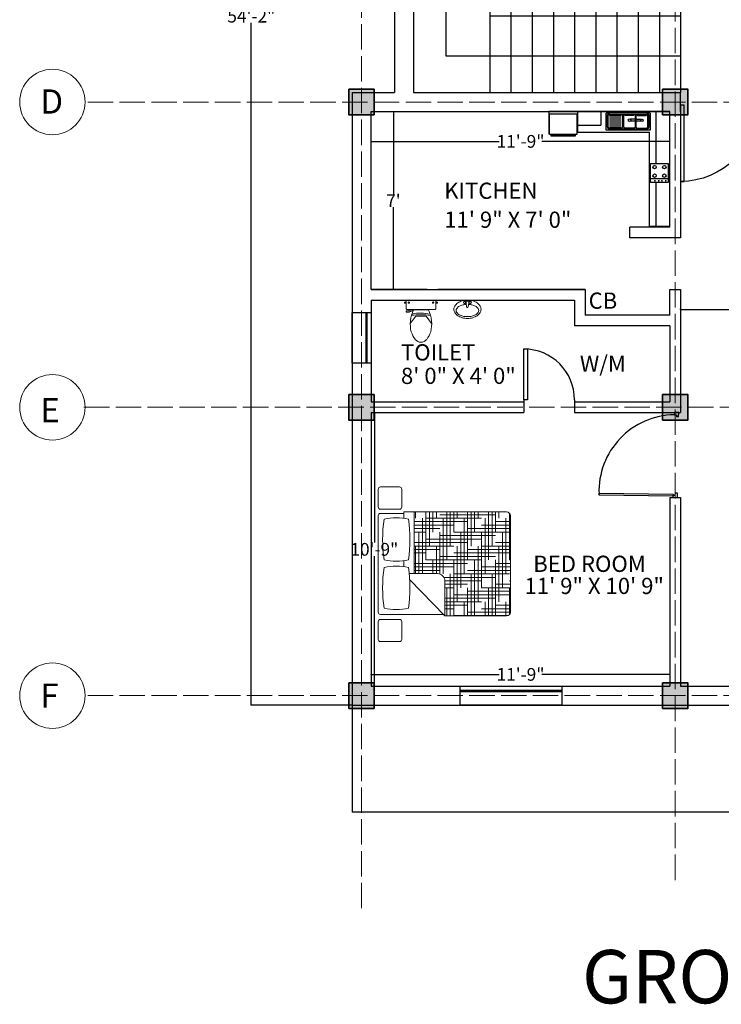
# Model space of a CAD drawing. Units: inches. Extents: x -113 to 5399, y -1393 to 3302.
# Tile 31 of 40: x 3074 to 3405, y 2439 to 2903. Entities that reach past the tile are written whole.
import ezdxf

# ---------------------------------------------------------------- set-up
doc = ezdxf.new("R2010")
doc.units = ezdxf.units.IN
doc.header["$MEASUREMENT"] = 0
doc.linetypes.add('ACAD_ISO02W100', pattern=[15, 12, -3])
for name, color, linetype, lineweight in [('A-ANNO-DIMS', 254, 'Continuous', 18), ('A-ANNO-TEXT', 7, 'Continuous', 25), ('A-AREA-IDEN', 4, 'Continuous', 18), ('A-COLS', 7, 'Continuous', 35), ('A-FLOR-CASE', 8, 'Continuous', 18), ('A-FLOR-FIXT', 8, 'Continuous', 18), ('A-GRID-IDEN', 7, 'Continuous', 18), ('doors', 2, 'Continuous', 25), ('DT TEXT', 4, 'Continuous', 18), ('furniture', 131, 'Continuous', 18), ('GRIDS', 7, 'ACAD_ISO02W100', 13), ('stairs', 210, 'Continuous', 25), ('walls', 1, 'Continuous', 25), ('windows', 3, 'Continuous', 25)]:
    doc.layers.add(name, color=color, linetype=linetype, lineweight=lineweight)
doc.layers.add('TEFRIŞ', color=11, linetype='Continuous')
doc.styles.get("Standard").update_dxf_attribs({"font": 'arial.ttf'})
doc.dimstyles.get("Standard").update_dxf_attribs({"dimtxt": 6, "dimasz": 0.18, "dimexe": 0.18, "dimexo": 0.0625, "dimgap": 0.09, "dimtad": 0, "dimtih": 1, "dimtoh": 1, "dimdec": 1, "dimzin": 0, "dimdsep": 46, "dimlunit": 4, "dimtxsty": 'Standard', "dimblk": 'ARCHTICK', "dimcen": 0.09, "dimadec": 0, "dimazin": 0, "dimtfac": 1, "dimtdec": 1, "dimtofl": 0, "dimtmove": 0, "dimatfit": 3, "dimfxl": 1, "dimtolj": 1, "dimtzin": 0, "dimarcsym": 0})

# ---------------------------------------------------------------- blocks, each defined once
blk = doc.blocks.new('*U2')
for p, q in [((0, 0), (0, -6)), ((24, 0), (24, -6))]:
    blk.add_line(p, q)
blk.add_lwpolyline([(0, 0), (0, 24), (1.75, 24), (1.75, 0)], close=True)
blk.add_arc((0, 0), 24, 0, 90)
blk = doc.blocks.new('*U3')
for p, q in [((0, 0), (0, -6)), ((36, 0), (36, -6))]:
    blk.add_line(p, q)
blk.add_lwpolyline([(0, 0), (0, 36), (1.75, 36), (1.75, 0)], close=True)
blk.add_arc((0, 0), 36, 0, 90)
blk = doc.blocks.new('*X4')
at = {"color": 0}
for p, q in [((4.359, 18.562), (4.359, 18.646)), ((4.5, 18), (4.5, 18.646)), ((4.547, 18.188), (4.547, 18.646)), ((4.594, 18.375), (4.594, 18.646)), ((4.641, 18.562), (4.641, 18.646)), ((4.687, 18.609), (5.437, 18.609)), ((4.781, 18), (4.781, 18.646)), ((4.828, 18.188), (4.828, 18.646)), ((4.875, 18.375), (4.875, 18.646)), ((4.922, 18.562), (4.922, 18.646)), ((5.062, 18), (5.062, 18.646)), ((5.109, 18.188), (5.109, 18.646)), ((5.156, 18.375), (5.156, 18.646)), ((5.203, 18.562), (5.203, 18.646)), ((5.344, 18), (5.344, 18.646)), ((5.391, 18.188), (5.391, 18.646)), ((5.437, 18.375), (5.437, 18.646)), ((5.484, 18.562), (5.484, 18.646)), ((5.625, 18), (5.625, 18.629)), ((4.34, 18.516), (5.062, 18.516)), ((4.34, 18.469), (4.875, 18.469)), ((4.453, 17.817), (4.453, 18.562)), ((4.5, 18.562), (5.25, 18.562)), ((4.734, 17.812), (4.734, 18.562)), ((5.016, 17.812), (5.016, 18.562)), ((5.25, 18.469), (5.637, 18.469)), ((5.297, 17.812), (5.297, 18.562)), ((5.437, 18.516), (5.637, 18.516)), ((5.578, 17.812), (5.578, 18.562)), ((5.625, 18.562), (5.637, 18.562)), ((4.34, 18.422), (4.687, 18.422)), ((4.34, 18.375), (4.5, 18.375)), ((4.406, 17.817), (4.406, 18.375)), ((4.687, 18.328), (5.437, 18.328)), ((4.687, 17.811), (4.687, 18.375)), ((4.875, 18.375), (5.625, 18.375)), ((4.969, 17.625), (4.969, 18.375)), ((5.062, 18.422), (5.637, 18.422)), ((5.25, 17.625), (5.25, 18.375)), ((5.531, 17.625), (5.531, 18.375)), ((4.34, 18.234), (5.062, 18.234)), ((4.34, 18.188), (4.875, 18.188)), ((4.359, 17.817), (4.359, 18.188)), ((4.5, 18.281), (5.25, 18.281)), ((4.641, 17.817), (4.641, 18.188)), ((4.922, 17.438), (4.922, 18.188)), ((5.203, 17.438), (5.203, 18.188)), ((5.25, 18.188), (5.637, 18.188)), ((5.437, 18.234), (5.637, 18.234)), ((5.484, 17.438), (5.484, 18.188)), ((5.625, 18.281), (5.637, 18.281)), ((4.34, 18.141), (4.687, 18.141)), ((4.34, 18.094), (4.5, 18.094)), ((4.687, 18.047), (5.437, 18.047)), ((4.875, 18.094), (5.625, 18.094)), ((5.062, 18.141), (5.637, 18.141)), ((4.34, 17.953), (5.062, 17.953)), ((4.34, 17.906), (4.875, 17.906)), ((4.5, 18), (5.25, 18)), ((4.594, 17.817), (4.594, 18)), ((4.875, 17.25), (4.875, 18)), ((5.156, 17.25), (5.156, 18)), ((5.25, 17.906), (5.637, 17.906)), ((5.437, 17.953), (5.637, 17.953)), ((5.437, 17.25), (5.437, 18)), ((5.625, 18), (5.637, 18)), ((4.34, 17.859), (4.687, 17.859)), ((4.828, 17.246), (4.828, 17.812)), ((4.875, 17.812), (5.625, 17.812)), ((5.062, 17.859), (5.637, 17.859)), ((5.109, 17.246), (5.109, 17.812)), ((5.391, 17.246), (5.391, 17.812)), ((4.742, 17.766), (5.437, 17.766)), ((4.755, 17.719), (5.25, 17.719)), ((4.755, 17.672), (5.062, 17.672)), ((5.437, 17.672), (5.637, 17.672)), ((5.625, 17.719), (5.637, 17.719)), ((4.755, 17.625), (4.875, 17.625)), ((4.781, 17.246), (4.781, 17.625)), ((4.875, 17.531), (5.625, 17.531)), ((5.062, 17.246), (5.062, 17.625)), ((5.062, 17.578), (5.637, 17.578)), ((5.25, 17.625), (5.637, 17.625)), ((5.344, 17.246), (5.344, 17.625)), ((5.625, 17.263), (5.625, 17.625)), ((4.755, 17.484), (5.437, 17.484)), ((4.755, 17.438), (5.25, 17.438)), ((4.755, 17.391), (5.062, 17.391)), ((5.016, 17.246), (5.016, 17.438)), ((5.297, 17.246), (5.297, 17.438)), ((5.437, 17.391), (5.637, 17.391)), ((5.578, 17.246), (5.578, 17.438)), ((5.625, 17.438), (5.637, 17.438)), ((4.755, 17.344), (4.875, 17.344)), ((4.875, 17.25), (5.608, 17.25)), ((4.969, 17.246), (4.969, 17.25)), ((5.062, 17.297), (5.637, 17.297)), ((5.25, 17.344), (5.637, 17.344)), ((5.25, 17.246), (5.25, 17.25)), ((5.531, 17.246), (5.531, 17.25))]:
    blk.add_line(p, q, dxfattribs=at)
blk = doc.blocks.new('MAT-P01')
for p, q in [((-0.021, 0.816), (-0.021, 0.56)), ((0.009, 0.846), (0.247, 0.846)), ((0.277, 0.816), (0.277, 0.56)), ((0.344, 0.816), (0.344, -0.032)), ((0.374, 0.846), (1.674, 0.846)), ((1.704, 0.816), (1.704, 0.5)), ((1.762, 0.816), (1.762, 0.56)), ((1.792, 0.846), (2.031, 0.846)), ((2.061, 0.816), (2.061, 0.56)), ((0.009, 0.53), (0.247, 0.53)), ((1.792, 0.53), (2.031, 0.53)), ((0.815, 0.423), (0.324, -0.051)), ((0.895, 0.429), (0.895, 0.049)), ((0.988, 0.5), (1.069, 0.5)), ((1.639, 0.5), (1.724, 0.5)), ((1.724, 0.5), (1.724, -0.884)), ((0.895, 0.364), (1.724, 0.364)), ((0.895, 0.364), (0.895, 0.049)), ((0.895, 0.364), (1.724, 0.364)), ((1.724, 0.364), (1.724, -0.884)), ((0.324, -0.051), (0.795, -0.051)), ((0.324, -0.051), (0.324, -0.884)), ((0.374, -0.934), (1.674, -0.934))]:
    blk.add_line(p, q)
for centre, radius, start, end in [((0.009, 0.816), 0.03, 90, 180), ((0.247, 0.816), 0.03, 0, 90), ((0.374, 0.816), 0.03, 90, 180), ((1.674, 0.816), 0.03, 0, 90), ((1.792, 0.816), 0.03, 90, 180), ((2.031, 0.816), 0.03, 0, 90), ((1.225, 0.603), 0.814, 168.373, 191.627), ((0.703, -1.144), 1.931, 81.8162, 98.1838), ((0.181, 0.603), 0.814, 348.373, 11.627), ((1.877, 0.603), 0.814, 168.373, 191.627), ((1.354, -1.144), 1.931, 81.8162, 98.1838), ((0.832, 0.603), 0.814, 348.373, 11.627), ((0.009, 0.56), 0.03, 180, 270), ((0.247, 0.56), 0.03, 270, 0), ((1.792, 0.56), 0.03, 180, 270), ((2.031, 0.56), 0.03, 270, 0), ((0.703, 2.35), 1.931, 261.8162, 278.1838), ((1.354, 2.35), 1.931, 261.8162, 278.1838), ((0.795, 0.049), 0.1, 270, 0), ((0.374, -0.884), 0.05, 180, 270), ((1.674, -0.884), 0.05, 270, 0)]:
    blk.add_arc(centre, radius, start, end)
at = {"rotation": 270}
blk.add_blockref('*X4', (-16.922, 4.704), dxfattribs=at)
blk = doc.blocks.new('A$C008029BD')
at = {"layer": 'TEFRIŞ', "ltscale": 0.05}
for p, q in [((0, 0), (0, -3.55)), ((3.37, 0), (0, 0)), ((3.37, 0), (3.37, -0.6)), ((1.522, -0.4), (0, -0.4)), ((3.37, -0.4), (2.083, -0.4)), ((0.05, -0.581), (0.05, -1.869)), ((0.05, -0.581), (0.55, -0.581)), ((0.086, -1.773), (0.086, -0.677)), ((0.096, -0.617), (0.454, -0.617)), ((0.099, -0.659), (0.457, -0.659)), ((0.113, -0.954), (0.113, -0.695)), ((0.23, -0.846), (0.229, -0.967)), ((0.28, -0.846), (0.277, -1.158)), ((0.493, -0.695), (0.493, -0.954)), ((0.514, -0.677), (0.514, -1.773)), ((0.55, -0.581), (0.55, -1.869)), ((0.6, -2.71), (0.6, -0.6)), ((3.37, -0.6), (0.6, -0.6)), ((0.096, -1.024), (0.454, -1.024)), ((0.457, -0.99), (0.099, -0.99)), ((0.11, -1.319), (0.11, -1.06)), ((0.228, -1.02), (0.227, -1.159)), ((0.49, -1.06), (0.49, -1.319)), ((0.454, -1.355), (0.096, -1.355)), ((0.096, -1.391), (0.454, -1.391)), ((0.11, -1.773), (0.11, -1.427)), ((0.154, -1.773), (0.154, -1.427)), ((0.214, -1.773), (0.214, -1.427)), ((0.274, -1.773), (0.274, -1.427)), ((0.334, -1.773), (0.334, -1.427)), ((0.39, -1.773), (0.39, -1.427)), ((0.444, -1.773), (0.444, -1.427)), ((0.49, -1.427), (0.49, -1.773)), ((0.55, -1.869), (0.05, -1.869)), ((0.454, -1.809), (0.096, -1.809)), ((0.454, -1.833), (0.096, -1.833)), ((0, -2.025), (0.4, -2.025)), ((0.4, -2.71), (0.4, -2.025)), ((0, -2.71), (0.6, -2.71)), ((0, -3.55), (0.65, -3.55))]:
    blk.add_line(p, q, dxfattribs=at)
at = {"layer": 'TEFRIŞ'}
blk.add_line((1.969, -0.05), (1.969, -0.572), dxfattribs=at)
at = {"layer": 'TEFRIŞ', "ltscale": 0.05}
for points in [[(1.522, -0.05), (2.083, -0.05), (2.083, -0.572), (1.522, -0.572)], [(0.67, -2.73), (0.67, -3.53), (0.07, -3.53), (0.07, -2.73)], [(0.72, -2.78), (0.72, -3.48), (0.67, -3.48), (0.67, -2.78)]]:
    blk.add_lwpolyline(points, close=True, dxfattribs=at)
at = {"layer": 'TEFRIŞ', "const_width": 0.025}
for points in [[(2.014, -0.123, 1), (2.039, -0.123, 1)], [(2.014, -0.236, 1), (2.039, -0.236, 1)], [(2.014, -0.327, 1), (2.039, -0.327, 1)], [(2.014, -0.44, 1), (2.039, -0.44, 1)]]:
    blk.add_lwpolyline(points, format="xyb", close=True, dxfattribs=at)
at = {"layer": 'TEFRIŞ', "ltscale": 0.05}
for centre, radius in [((1.628, -0.164), 0.0505), ((1.628, -0.45), 0.0505), ((0.255, -0.82), 0.036), ((0.252, -1.184), 0.036)]:
    blk.add_circle(centre, radius, dxfattribs=at)
at = {"layer": 'TEFRIŞ'}
for centre in [(1.88, -0.164), (1.88, -0.45)]:
    blk.add_circle(centre, 0.0505, dxfattribs=at)
at = {"layer": 'TEFRIŞ', "ltscale": 0.05}
for centre, radius, start, end in [((0.108, -0.649), 0.0351, 110.4976, 230.5777), ((0.118, -0.673), 0.023, 143.9853, 258.5157), ((0.454, -0.677), 0.06, 0, 90), ((0.457, -0.695), 0.036, 0, 90), ((0.115, -1.038), 0.023, 143.9853, 258.5157), ((0.118, -0.976), 0.023, 101.4843, 216.0147), ((0.454, -1.06), 0.036, 0, 90), ((0.457, -0.954), 0.036, 270, 0), ((0.115, -1.341), 0.023, 101.4843, 216.0147), ((0.115, -1.405), 0.023, 143.9853, 258.5157), ((0.454, -1.319), 0.036, 270, 0), ((0.454, -1.427), 0.036, 0, 90), ((0.108, -1.801), 0.0351, 129.4223, 249.5024), ((0.115, -1.796), 0.023, 101.4843, 216.0147), ((0.454, -1.773), 0.06, 270, 0), ((0.454, -1.773), 0.036, 270, 0)]:
    blk.add_arc(centre, radius, start, end, dxfattribs=at)
blk = doc.blocks.new('toilet-3')
at = {"color": 0, "linetype": 'ByBlock'}
for p, q in [((-0.281, -0.05), (-0.281, -0.069)), ((-0.281, -0.05), (-0.261, -0.05)), ((-0.281, -0.069), (-0.261, -0.069)), ((-0.261, -0.047), (-0.261, -0.072)), ((-0.261, -0.047), (-0.251, -0.047)), ((-0.261, -0.072), (-0.251, -0.072)), ((-0.251, -0.047), (-0.251, -0.072)), ((-0.25, -0.03), (-0.25, -0.165)), ((0.24, -0.02), (-0.24, -0.02)), ((0.25, -0.03), (0.25, -0.165)), ((0.261, -0.047), (0.251, -0.047)), ((0.251, -0.047), (0.251, -0.072)), ((0.261, -0.072), (0.251, -0.072)), ((0.261, -0.047), (0.261, -0.072)), ((0.281, -0.05), (0.261, -0.05)), ((0.281, -0.069), (0.261, -0.069)), ((0.281, -0.05), (0.281, -0.069)), ((-0.144, -0.2), (-0.25, -0.2)), ((-0.25, -0.2), (-0.25, -0.222)), ((-0.198, -0.222), (-0.25, -0.222)), ((0.24, -0.175), (-0.24, -0.175)), ((-0.202, -0.2), (-0.202, -0.175)), ((-0.198, -0.222), (-0.16, -0.207)), ((-0.089, -0.287), (-0.18, -0.415)), ((-0.16, -0.207), (-0.16, -0.2)), ((-0.144, -0.2), (-0.144, -0.175)), ((0.125, -0.182), (-0.125, -0.182)), ((0.089, -0.287), (-0.089, -0.287)), ((0.089, -0.287), (0.18, -0.415))]:
    blk.add_line(p, q, dxfattribs=at)
for centre in [(-0.205, -0.059), (0.205, -0.059)]:
    blk.add_circle(centre, 0.0125, dxfattribs=at)
for centre, radius, start, end in [((-0.24, -0.03), 0.01, 90, 180), ((-0.24, -0.165), 0.01, 180, 270), ((0.24, -0.03), 0.01, 0, 90), ((0.24, -0.165), 0.01, 270, 0), ((0.376, -0.424), 0.557, 154.2321, 193.6755), ((-0.013, -1.787), 1.521, 83.4552, 95.5271), ((-0.005, -0.896), 0.659, 75.9276, 103.0204), ((-0.376, -0.424), 0.557, 346.3245, 25.7679), ((0.262, -0.406), 0.452, 199.2942, 217.2549), ((-0.265, -0.4), 0.457, 322.2382, 340.1051), ((-0.001, -0.609), 0.12, 216.3794, 323.6206)]:
    blk.add_arc(centre, radius, start, end, dxfattribs=at)
blk = doc.blocks.new('wash-6')
at = {"color": 0, "linetype": 'ByBlock'}
for p, q in [((-0.036, -0.063), (-0.021, -0.18)), ((0.036, -0.063), (0.021, -0.18))]:
    blk.add_line(p, q, dxfattribs=at)
for centre, radius in [((-0.075, -0.062), 0.0325), ((-0.075, -0.062), 0.0263), ((0.075, -0.062), 0.0325), ((0.075, -0.062), 0.0263)]:
    blk.add_circle(centre, radius, dxfattribs=at)
for centre, radius, start, end in [((0, -0.56), 0.56, 90, 105.4371), ((-0.204, -0.25), 0.17, 148.1465, 180), ((-0.204, -0.25), 0.17, 180, 211.8535), ((-0.107, -0.311), 0.285, 123.6901, 148.1465), ((-0.217, -0.282), 0.0954, 142.5096, 180), ((-0.114, -0.361), 0.225, 118.369, 142.5096), ((-0.042, -0.407), 0.401, 105.4371, 123.6901), ((-0.045, -0.488), 0.37, 102.6081, 118.369), ((0, -0.69), 0.576, 92.9466, 102.6081), ((0, -0.063), 0.0361, 0, 180), ((0, -0.18), 0.0215, 180, 0), ((0, -0.56), 0.56, 74.5629, 90), ((0, -0.69), 0.576, 77.3919, 87.0534), ((0.045, -0.488), 0.37, 61.631, 77.3919), ((0.042, -0.407), 0.401, 56.3099, 74.5629), ((0.114, -0.361), 0.225, 37.4904, 61.631), ((0.107, -0.311), 0.285, 31.8535, 56.3099), ((0.217, -0.282), 0.0954, 0, 37.4904), ((0.204, -0.25), 0.17, 0, 31.8535), ((0.204, -0.25), 0.17, 328.1465, 0), ((-0.107, -0.189), 0.285, 211.8535, 236.3099), ((-0.217, -0.282), 0.0954, 180, 217.4904), ((-0.114, -0.203), 0.225, 217.4904, 241.631), ((-0.042, -0.092), 0.401, 236.3099, 254.5629), ((-0.045, -0.076), 0.37, 241.631, 257.3919), ((0, 0.06), 0.56, 254.5629, 270), ((0, 0.125), 0.576, 257.3919, 270), ((0, 0.125), 0.576, 270, 282.6081), ((0, 0.06), 0.56, 270, 285.4371), ((0.045, -0.076), 0.37, 282.6081, 298.369), ((0.042, -0.092), 0.401, 285.4371, 303.6901), ((0.114, -0.203), 0.225, 298.369, 322.5096), ((0.107, -0.189), 0.285, 303.6901, 328.1465), ((0.217, -0.282), 0.0954, 322.5096, 0)]:
    blk.add_arc(centre, radius, start, end, dxfattribs=at)
blk = doc.blocks.new('_ArchTick')
at = {"color": 0, "linetype": 'ByBlock', "const_width": 0.15}
blk.add_lwpolyline([(-0.5, -0.5), (0.5, 0.5)], dxfattribs=at)
blk = doc.blocks.new('*D129')
at = {"layer": 'A-ANNO-DIMS', "color": 0, "lineweight": -2, "transparency": 16777216}
for p, q in [((3230.55, 2580), (3230.55, 2529.62)), ((3663.55, 2580), (3663.55, 2529.62)), ((3230.55, 2529.8), (3436.65, 2529.8)), ((3663.55, 2529.8), (3457.44, 2529.8))]:
    blk.add_line(p, q, dxfattribs=at)
at = {"layer": 'Defpoints', "color": 0, "transparency": 16777216}
for p in [(3230.55, 2580.06), (3663.55, 2580.06), (3663.55, 2529.8)]:
    blk.add_point(p, dxfattribs=at)
at = {"layer": 'A-ANNO-DIMS', "color": 0, "lineweight": -2, "transparency": 16777216, "xscale": 0.18, "yscale": 0.18, "zscale": 0.18, "rotation": 180}
blk.add_blockref('_ArchTick', (3230.55, 2529.8), dxfattribs=at)
at = {"layer": 'A-ANNO-DIMS', "color": 0, "lineweight": -2, "transparency": 16777216, "xscale": 0.18, "yscale": 0.18, "zscale": 0.18}
blk.add_blockref('_ArchTick', (3663.55, 2529.8), dxfattribs=at)
at = {"layer": 'A-ANNO-DIMS', "color": 0, "transparency": 16777216, "insert": (3447.05, 2529.8), "char_height": 6, "attachment_point": 5}
blk.add_mtext('\\A1;36\'-1"', dxfattribs=at)
blk = doc.blocks.new('*D130')
at = {"layer": 'A-ANNO-DIMS', "color": 0, "lineweight": -2, "transparency": 16777216}
for p, q in [((3230.48, 3230.06), (3182.83, 3230.06)), ((3183.01, 3230.06), (3183.01, 2908.21)), ((3183.01, 2580.06), (3183.01, 2901.91)), ((3230.48, 2580.06), (3182.83, 2580.06))]:
    blk.add_line(p, q, dxfattribs=at)
at = {"layer": 'Defpoints', "color": 0, "transparency": 16777216}
for p in [(3230.55, 3230.06), (3183.01, 2580.06), (3230.55, 2580.06)]:
    blk.add_point(p, dxfattribs=at)
at = {"layer": 'A-ANNO-DIMS', "color": 0, "lineweight": -2, "transparency": 16777216, "xscale": 0.18, "yscale": 0.18, "zscale": 0.18}
for p, rotation in [((3183.01, 3230.06), 90), ((3183.01, 2580.06), 270)]:
    blk.add_blockref('_ArchTick', p, dxfattribs=dict(at, rotation=rotation))
at = {"layer": 'A-ANNO-DIMS', "color": 0, "transparency": 16777216, "insert": (3183.01, 2905.06), "char_height": 6, "attachment_point": 5}
blk.add_mtext('\\A1;54\'-2"', dxfattribs=at)
blk = doc.blocks.new('*D128')
at = {"layer": 'A-ANNO-DIMS', "color": 0, "lineweight": -2, "transparency": 16777216}
for p, q in [((3385.55, 2766.62), (3385.55, 2766.93)), ((3385.55, 2766.75), (3446.65, 2766.75)), ((3517.55, 2766.75), (3456.45, 2766.75)), ((3517.55, 2766.62), (3517.55, 2766.93))]:
    blk.add_line(p, q, dxfattribs=at)
at = {"layer": 'Defpoints', "color": 0, "transparency": 16777216}
for p in [(3385.55, 2766.75), (3385.55, 2766.56), (3517.55, 2766.56)]:
    blk.add_point(p, dxfattribs=at)
at = {"layer": 'A-ANNO-DIMS', "color": 0, "lineweight": -2, "transparency": 16777216, "xscale": 0.18, "yscale": 0.18, "zscale": 0.18, "rotation": 180}
blk.add_blockref('_ArchTick', (3385.55, 2766.75), dxfattribs=at)
at = {"layer": 'A-ANNO-DIMS', "color": 0, "lineweight": -2, "transparency": 16777216, "xscale": 0.18, "yscale": 0.18, "zscale": 0.18}
blk.add_blockref('_ArchTick', (3517.55, 2766.75), dxfattribs=at)
at = {"layer": 'A-ANNO-DIMS', "color": 0, "transparency": 16777216, "insert": (3451.55, 2766.75), "char_height": 6, "attachment_point": 5}
blk.add_mtext("\\A1;11'", dxfattribs=at)
blk = doc.blocks.new('*D136')
at = {"layer": 'A-ANNO-DIMS', "color": 0, "lineweight": -2, "transparency": 16777216}
for p, q in [((3248.98, 2860.06), (3250.22, 2860.06)), ((3250.04, 2860.06), (3250.04, 2821.15)), ((3250.04, 2776.06), (3250.04, 2814.97)), ((3248.98, 2776.06), (3250.22, 2776.06))]:
    blk.add_line(p, q, dxfattribs=at)
at = {"layer": 'Defpoints', "color": 0, "transparency": 16777216}
for p in [(3248.91, 2860.06), (3248.91, 2776.06), (3250.04, 2776.06)]:
    blk.add_point(p, dxfattribs=at)
at = {"layer": 'A-ANNO-DIMS', "color": 0, "lineweight": -2, "transparency": 16777216, "xscale": 0.18, "yscale": 0.18, "zscale": 0.18}
for p, rotation in [((3250.04, 2860.06), 90), ((3250.04, 2776.06), 270)]:
    blk.add_blockref('_ArchTick', p, dxfattribs=dict(at, rotation=rotation))
at = {"layer": 'A-ANNO-DIMS', "color": 0, "transparency": 16777216, "insert": (3250.04, 2818.06), "char_height": 6, "attachment_point": 5}
blk.add_mtext("\\A1;7'", dxfattribs=at)
blk = doc.blocks.new('*D137')
at = {"layer": 'A-ANNO-DIMS', "color": 0, "lineweight": -2, "transparency": 16777216}
for p, q in [((3239.55, 2846.05), (3239.55, 2846.17)), ((3239.55, 2845.99), (3299.93, 2845.99)), ((3380.55, 2845.99), (3320.16, 2845.99)), ((3380.55, 2846.05), (3380.55, 2846.17))]:
    blk.add_line(p, q, dxfattribs=at)
at = {"layer": 'Defpoints', "color": 0, "transparency": 16777216}
for p in [(3239.55, 2845.99), (3380.55, 2845.99), (3380.55, 2845.99)]:
    blk.add_point(p, dxfattribs=at)
at = {"layer": 'A-ANNO-DIMS', "color": 0, "lineweight": -2, "transparency": 16777216, "xscale": 0.18, "yscale": 0.18, "zscale": 0.18, "rotation": 180}
blk.add_blockref('_ArchTick', (3239.55, 2845.99), dxfattribs=at)
at = {"layer": 'A-ANNO-DIMS', "color": 0, "lineweight": -2, "transparency": 16777216, "xscale": 0.18, "yscale": 0.18, "zscale": 0.18}
blk.add_blockref('_ArchTick', (3380.55, 2845.99), dxfattribs=at)
at = {"layer": 'A-ANNO-DIMS', "color": 0, "transparency": 16777216, "insert": (3310.05, 2845.99), "char_height": 6, "attachment_point": 5}
blk.add_mtext('\\A1;11\'-9"', dxfattribs=at)
blk = doc.blocks.new('*D138')
at = {"layer": 'A-ANNO-DIMS', "color": 0, "lineweight": -2, "transparency": 16777216}
for p, q in [((3240.53, 2718.06), (3241.25, 2718.06)), ((3241.07, 2718.06), (3241.07, 2656.71)), ((3241.07, 2589.06), (3241.07, 2650.41)), ((3240.53, 2589.06), (3241.25, 2589.06))]:
    blk.add_line(p, q, dxfattribs=at)
at = {"layer": 'Defpoints', "color": 0, "transparency": 16777216}
for p in [(3240.47, 2718.06), (3240.47, 2589.06), (3241.07, 2589.06)]:
    blk.add_point(p, dxfattribs=at)
at = {"layer": 'A-ANNO-DIMS', "color": 0, "lineweight": -2, "transparency": 16777216, "xscale": 0.18, "yscale": 0.18, "zscale": 0.18}
for p, rotation in [((3241.07, 2718.06), 90), ((3241.07, 2589.06), 270)]:
    blk.add_blockref('_ArchTick', p, dxfattribs=dict(at, rotation=rotation))
at = {"layer": 'A-ANNO-DIMS', "color": 0, "transparency": 16777216, "insert": (3241.07, 2653.56), "char_height": 6, "attachment_point": 5}
blk.add_mtext('\\A1;10\'-9"', dxfattribs=at)
blk = doc.blocks.new('*D139')
at = {"layer": 'A-ANNO-DIMS', "color": 0, "lineweight": -2, "transparency": 16777216}
for p, q in [((3239.55, 2594.5), (3239.55, 2594.74)), ((3239.55, 2594.56), (3299.93, 2594.56)), ((3380.55, 2594.56), (3320.16, 2594.56)), ((3380.55, 2594.5), (3380.55, 2594.74))]:
    blk.add_line(p, q, dxfattribs=at)
at = {"layer": 'Defpoints', "color": 0, "transparency": 16777216}
for p in [(3239.55, 2594.56), (3239.55, 2594.44), (3380.55, 2594.44)]:
    blk.add_point(p, dxfattribs=at)
at = {"layer": 'A-ANNO-DIMS', "color": 0, "lineweight": -2, "transparency": 16777216, "xscale": 0.18, "yscale": 0.18, "zscale": 0.18, "rotation": 180}
blk.add_blockref('_ArchTick', (3239.55, 2594.56), dxfattribs=at)
at = {"layer": 'A-ANNO-DIMS', "color": 0, "lineweight": -2, "transparency": 16777216, "xscale": 0.18, "yscale": 0.18, "zscale": 0.18}
blk.add_blockref('_ArchTick', (3380.55, 2594.56), dxfattribs=at)
at = {"layer": 'A-ANNO-DIMS', "color": 0, "transparency": 16777216, "insert": (3310.05, 2594.56), "char_height": 6, "attachment_point": 5}
blk.add_mtext('\\A1;11\'-9"', dxfattribs=at)
blk = doc.blocks.new('WIN-PLAN-48IN')
h = blk.add_hatch(color=256)
h.dxf.hatch_style = 1
h.paths.add_polyline_path([(48, 2.5), (0, 2.5), (0, 2), (48, 2)])
for p, q in [((0, 9), (48, 9)), ((0, 0), (0, 9)), ((48, 9), (48, 0)), ((48, 2.5), (0, 2.5)), ((48, 2), (0, 2)), ((48, 0), (0, 0))]:
    blk.add_line(p, q)
blk = doc.blocks.new('WIN-PLAN-24IN')
h = blk.add_hatch(color=256)
h.dxf.hatch_style = 1
h.paths.add_polyline_path([(6.5, 24), (6.5, 0), (7, 0), (7, 24)])
for p, q in [((0, 0), (0, 24)), ((0, 24), (9, 24)), ((6.5, 24), (6.5, 0)), ((7, 24), (7, 0)), ((9, 24), (9, 0)), ((9, 0), (0, 0))]:
    blk.add_line(p, q)
blk = doc.blocks.new('COLUMN-12IN-SQUARE')
h = blk.add_hatch(color=256)
h.dxf.hatch_style = 1
h.paths.add_polyline_path([(6, 6), (-6, 6), (-6, -6), (6, -6)])
blk.add_lwpolyline([(-6, 6), (6, 6), (6, -6), (-6, -6)], close=True)
blk = doc.blocks.new('STAIR-RESIDENTIAL-PLAN')
for p, q in [((20.54, 72), (20.54, 0)), ((30.54, 72), (30.54, 0)), ((40.54, 72), (40.54, 0)), ((50.54, 72), (50.54, 0)), ((60.54, 72), (60.54, 0)), ((70.54, 72), (70.54, 0)), ((80.54, 72), (80.54, 0)), ((90.54, 72), (90.54, 0)), ((100.54, 72), (100.54, 0)), ((110.54, 72), (110.54, 0)), ((110.54, 54.14), (107.61, 56.9)), ((107.61, 56.9), (107.61, 54.14)), ((0, 17.09), (0, 54.14)), ((0, 54.14), (107.61, 54.14)), ((110.54, 54.14), (107.61, 51.38)), ((107.61, 51.38), (107.61, 54.14)), ((110.54, 36), (20.54, 36)), ((110.54, 17.09), (0, 17.09))]:
    blk.add_line(p, q)
blk = doc.blocks.new('DOOR-SINGLE-36IN-PLAN')
for p, q in [((0.5, 2), (0.5, 36.98)), ((0.5, 36.98), (1.5, 36.98)), ((1.5, 36.98), (1.5, 2)), ((0, 2), (0, 0)), ((0, 2), (1.04, 2)), ((1.5, 2), (0.5, 2)), ((1.04, 2), (1.04, 0.98)), ((1.04, 0.98), (2, 0.98)), ((2, 0), (2, 0.98)), ((38.96, 0.98), (38, 0.98)), ((38, 0), (38, 0.98)), ((40, 2), (38.96, 2)), ((38.96, 2), (38.96, 0.98)), ((40, 0), (40, 2)), ((0, 0), (2, 0)), ((0, 0), (2, 0)), ((38, 0), (40, 0))]:
    blk.add_line(p, q)
blk.add_arc((2.94, 0.99), 36.04, 1.6003, 93.0893)
blk = doc.blocks.new('GRID-BUBBLE-D')
blk.add_circle((0, 0), 15.44)
blk.add_text('D', height=11.45).set_placement((-5.69, -5.49))
blk = doc.blocks.new('GRID-BUBBLE-E')
blk.add_circle((0, 0), 15.44)
blk.add_text('E', height=11.45).set_placement((-5.69, -7.06))
blk = doc.blocks.new('GRID-BUBBLE-F')
blk.add_circle((0, 0), 15.44)
blk.add_text('F', height=11.45).set_placement((-5.69, -5.75))

msp = doc.modelspace()

# ---------------------------------------------------------------- linework, layer by layer
at = {"layer": 'GRIDS'}
for p, q in [((3234.97, 3261.26), (3234.97, 2482.84)), ((3383.05, 2497.57), (3383.05, 3256.61)), ((3762.86, 2864.56), (3104.61, 2864.56)), ((3104.07, 2720.56), (3762.86, 2720.56)), ((3762.86, 2584.56), (3104.61, 2584.56))]:
    msp.add_line(p, q, dxfattribs=at)
at = {"layer": 'walls'}
for p, q in [((3250.55, 2941.06), (3250.55, 2869.06)), ((3259.55, 2941.06), (3259.55, 2869.06)), ((3230.55, 2869.06), (3230.55, 2580.06)), ((3230.55, 2869.06), (3250.55, 2869.06)), ((3259.55, 2869.06), (3385.55, 2869.06)), ((3385.55, 2860.06), (3385.55, 2869.06)), ((3239.55, 2860.06), (3323.4, 2860.06)), ((3239.55, 2776.06), (3239.55, 2860.06)), ((3271.05, 2860.06), (3380.55, 2860.06)), ((3380.55, 2805.56), (3380.55, 2860.06)), ((3385.55, 2860.06), (3385.55, 2800.56)), ((3380.55, 2805.56), (3361.55, 2805.56)), ((3361.55, 2800.56), (3361.55, 2805.56)), ((3385.55, 2800.56), (3361.55, 2800.56)), ((3266.05, 2776.06), (3239.55, 2776.06)), ((3239.55, 2776.06), (3266.05, 2776.06)), ((3266.05, 2776.06), (3271.05, 2776.06)), ((3340.55, 2776.06), (3271.05, 2776.06)), ((3271.05, 2776.06), (3340.55, 2776.06)), ((3340.55, 2776.06), (3340.55, 2764.06)), ((3380.55, 2764.06), (3380.55, 2776.06)), ((3380.55, 2776.06), (3385.55, 2776.06)), ((3385.55, 2776.06), (3385.55, 2718.06)), ((3239.55, 2771.06), (3239.55, 2723.06)), ((3239.55, 2771.06), (3335.55, 2771.06)), ((3239.55, 2771.06), (3335.55, 2771.06)), ((3335.55, 2771.06), (3335.55, 2759.06)), ((3380.55, 2764.06), (3340.55, 2764.06)), ((3380.55, 2759.06), (3335.55, 2759.06)), ((3380.55, 2759.06), (3380.55, 2723.06)), ((3239.55, 2723.06), (3311.55, 2723.06)), ((3311.55, 2723.06), (3311.55, 2718.06)), ((3335.55, 2724.06), (3335.55, 2718.06)), ((3335.55, 2723.06), (3380.55, 2723.06)), ((3239.55, 2718.06), (3239.55, 2589.06)), ((3239.55, 2718.06), (3311.55, 2718.06)), ((3335.55, 2718.06), (3380.55, 2718.06)), ((3380.55, 2718.06), (3385.55, 2718.06)), ((3380.55, 2678.06), (3380.55, 2589.06)), ((3380.55, 2678.06), (3385.55, 2678.06)), ((3385.55, 2678.06), (3385.55, 2589.06)), ((3239.55, 2589.06), (3380.55, 2589.06)), ((3385.55, 2589.06), (3427.55, 2589.06)), ((3230.55, 2580.06), (3427.55, 2580.06))]:
    msp.add_line(p, q, dxfattribs=at)

# ---------------------------------------------------------------- block references
at = {"layer": 'A-COLS'}
for p in [(3234.97, 2864.56), (3383.05, 2864.56), (3234.97, 2720.56), (3383.05, 2720.56), (3234.97, 2584.56), (3383.05, 2584.56)]:
    msp.add_blockref('COLUMN-12IN-SQUARE', p, dxfattribs=at)
at = {"layer": 'A-FLOR-CASE', "xscale": 16.09806929200166, "yscale": 16.09806929200166, "zscale": 16.09806929200166, "rotation": 270}
msp.add_blockref('A$C008029BD', (3380.55, 2860.06), dxfattribs=at)
at = {"layer": 'A-FLOR-FIXT'}
for name, p, xscale, yscale, zscale in [('toilet-3', (3263.08, 2771.62), 27.95492935005888, 27.95492935005888, 27.95492935005888), ('wash-6', (3284.99, 2771.06), 17.16666334294967, 17.16666334294967, 17.16666334294967)]:
    msp.add_blockref(name, p, dxfattribs=dict(at, xscale=xscale, yscale=yscale, zscale=zscale))
at = {"layer": 'A-GRID-IDEN'}
for name, p in [('GRID-BUBBLE-D', (3089.17, 2864.56)), ('GRID-BUBBLE-E', (3089.17, 2720.56)), ('GRID-BUBBLE-F', (3089.17, 2584.56))]:
    msp.add_blockref(name, p, dxfattribs=at)
at = {"layer": 'doors', "xscale": -1, "rotation": 180}
msp.add_blockref('*U3', (3385.55, 2863.06), dxfattribs=at)
at = {"layer": 'doors'}
msp.add_blockref('*U2', (3311.55, 2724.06), dxfattribs=at)
at = {"layer": 'doors', "rotation": 89.09244041658943}
msp.add_blockref('DOOR-SINGLE-36IN-PLAN', (3384.05, 2678.04), dxfattribs=at)
at = {"layer": 'furniture', "xscale": 35.02364872074636, "yscale": 35.02364872074636, "zscale": 35.02364872074636, "rotation": 90}
msp.add_blockref('MAT-P01', (3272.54, 2610.79), dxfattribs=at)
at = {"layer": 'stairs'}
msp.add_blockref('STAIR-RESIDENTIAL-PLAN', (3275.01, 2869.06), dxfattribs=at)
at = {"layer": 'windows'}
msp.add_blockref('WIN-PLAN-24IN', (3230.55, 2741.34), dxfattribs=at)
at = {"layer": 'windows', "rotation": 180}
msp.add_blockref('WIN-PLAN-48IN', (3329.55, 2589.06), dxfattribs=at)

# ---------------------------------------------------------------- texts
at = {"layer": 'A-ANNO-TEXT'}
msp.add_text('GROUND FLOOR', height=25.17, dxfattribs=at).set_placement((3339.05, 2439.4))
at = {"layer": 'A-AREA-IDEN'}
for s, height, p in [('KITCHEN', 7.647, (3274.06, 2818.89)), ('11\' 9" X 7\' 0"', 7.6473, (3274.06, 2805.21)), ('TOILET', 7.647, (3253.63, 2742.65)), ('8\' 0" X 4\' 0"', 7.6473, (3253.63, 2731.57)), ('BED ROOM', 7.647, (3316.05, 2642.91)), ('11\' 9" X 10\' 9"', 7.6473, (3311.95, 2632.49))]:
    msp.add_text(s, height=height, dxfattribs=at).set_placement(p)
at = {"layer": 'DT TEXT'}
for s, p in [('CB', (3342.17, 2767.04)), (' W/M', (3335.7, 2737.29))]:
    msp.add_text(s, height=7.647, dxfattribs=at).set_placement(p)

# ---------------------------------------------------------------- dimensions: what is measured, and where the dimension line sits
at = {"layer": 'A-ANNO-DIMS'}
for base, p1, p2, picture, middle in [((3183.01, 2580.06), (3230.55, 3230.06), (3230.55, 2580.06), '*D130', (3183.01, 2905.06)), ((3250.04, 2776.06), (3248.91, 2860.06), (3248.91, 2776.06), '*D136', (3250.04, 2818.06)), ((3241.07, 2589.06), (3240.47, 2718.06), (3240.47, 2589.06), '*D138', (3241.07, 2653.56))]:
    dim = msp.add_linear_dim(base=base, p1=p1, p2=p2, angle=90, dimstyle='Standard', override={"dimclrd": 0, "dimclre": 0, "dimclrt": 0}, dxfattribs=at)
    dim.commit()
    dim.dimension.update_dxf_attribs({"geometry": picture, "text_midpoint": middle})
for base, p1, p2, picture, middle in [((3380.55, 2845.99), (3239.55, 2845.99), (3380.55, 2845.99), '*D137', (3310.05, 2845.99)), ((3385.55, 2766.75), (3517.55, 2766.56), (3385.55, 2766.56), '*D128', (3451.55, 2766.75)), ((3239.55, 2594.56), (3380.55, 2594.44), (3239.55, 2594.44), '*D139', (3310.05, 2594.56)), ((3663.55, 2529.8), (3230.55, 2580.06), (3663.55, 2580.06), '*D129', (3447.05, 2529.8))]:
    dim = msp.add_linear_dim(base=base, p1=p1, p2=p2, dimstyle='Standard', override={"dimclrd": 0, "dimclre": 0, "dimclrt": 0}, dxfattribs=at)
    dim.commit()
    dim.dimension.update_dxf_attribs({"geometry": picture, "text_midpoint": middle})

doc.saveas('drawing.dxf')
